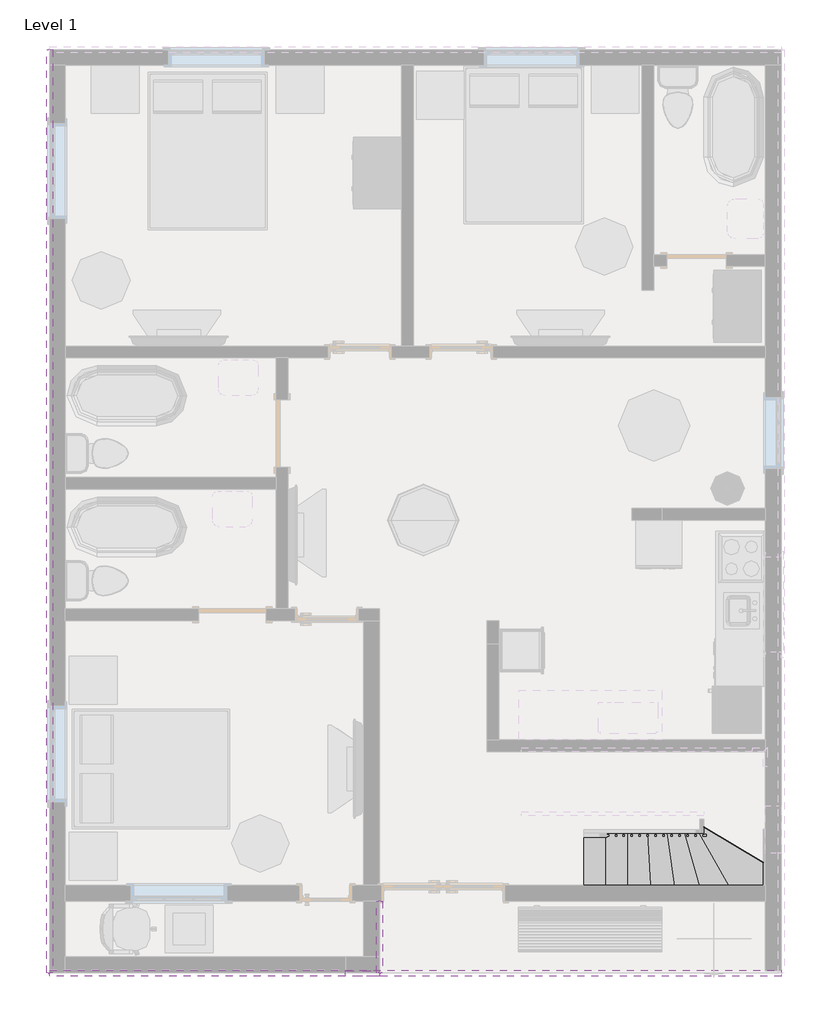
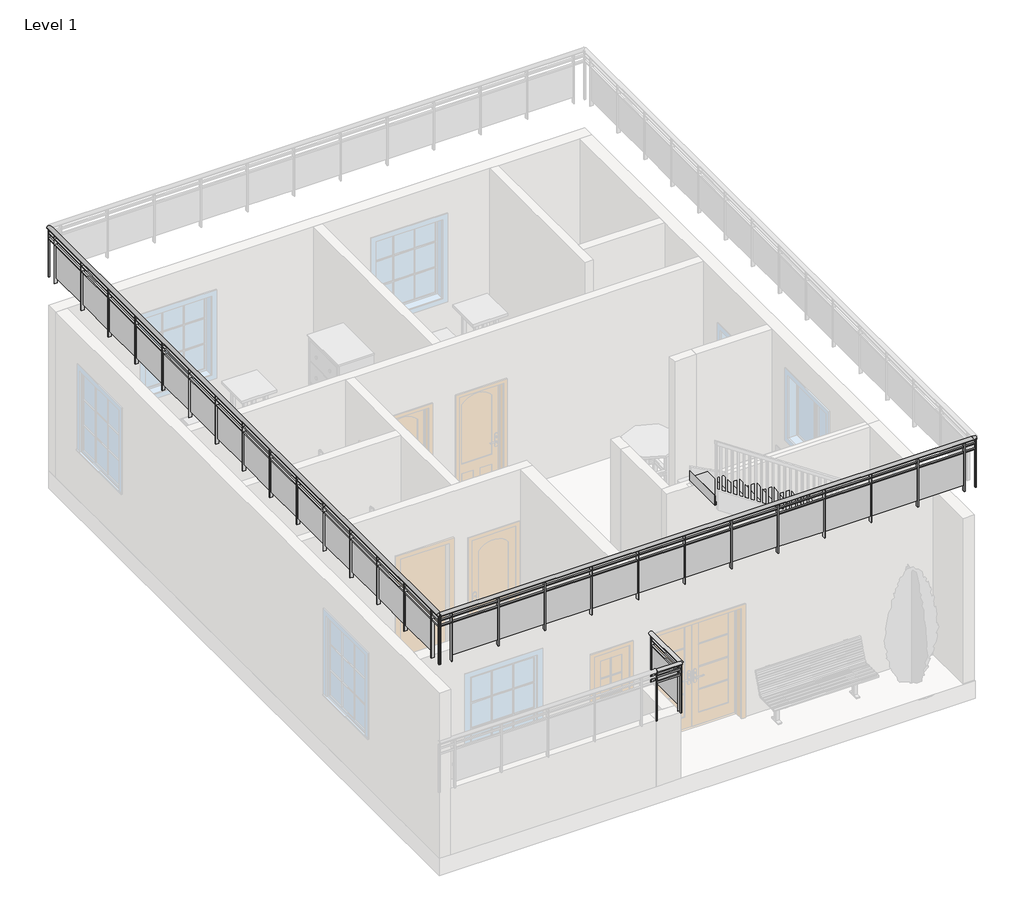
# One storey, part 2 of 4: 4 railings, 1 stair flight.
"""IFC4 building model written with IfcOpenShell, lengths in millimetres."""

from ifc_helpers import new_model, si_unit, point, frame, origin, place, context, project, spatial, polyline, ellipse_curve, trimmed, outline, extrude, transform, mapped, element, save
from ifc_brep_helpers import plane_surface, extruded_surface, advanced_brep
from components import stair_flight_7608b1ce

model = new_model("IFC4")

# Units and contexts
model_context = context("Model", 3, world=origin())
ifc_project = project(units=[si_unit("LENGTHUNIT", "METRE", prefix="MILLI")], contexts=[model_context])

# Site, building, storey
site = spatial("IfcSite", under=ifc_project)
building = spatial("IfcBuilding", under=site)
storey = spatial("IfcBuildingStorey", under=building, Name="Level 1", Elevation=0.0)

# Railings
placement = place(None, origin())
element("IfcRailing", 1, ObjectType="Glass Panel - Bottom Fill", at=placement, inside=storey, context=model_context, shape_type="SolidModel", body=[
    advanced_brep(
    [(-20.3394177, -1651.5409676, 2133.6), (-20.3394177, -1727.7409676, 2133.6), (411.4605823, -1651.5409676, 2133.6), (411.4605823, -1727.7409676, 2133.6)],
    [
        (0, 1, ellipse_curve(frame((-20.3394177, -1689.6409676, 2133.6), z_axis=(-1.0, 0.0, 0.0), x_axis=(0.0, -1.0, 0.0)), 38.1, 28.575)),
        (1, 0, ellipse_curve(frame((-20.3394177, -1689.6409676, 2133.6), z_axis=(-1.0, 0.0, 0.0), x_axis=(0.0, -1.0, 0.0)), 38.1, 28.575)),
        (2, 3, ellipse_curve(frame((411.4605823, -1689.6409676, 2133.6), z_axis=(1.0, 0.0, 0.0), x_axis=(0.0, -1.0, 0.0)), 38.1, 28.575)),
        (3, 2, ellipse_curve(frame((411.4605823, -1689.6409676, 2133.6), z_axis=(1.0, 0.0, 0.0), x_axis=(0.0, -1.0, 0.0)), 38.1, 28.575)),
        (0, 2),
        (3, 1),
    ],
    [
        plane_surface(frame((-20.3394177, -1689.6409676, 2133.6), z_axis=(-1.0, 0.0, 0.0), x_axis=(0.0, 1.0, 0.0))),
        plane_surface(frame((411.4605823, -1689.6409676, 2133.6), z_axis=(1.0, 0.0, 0.0), x_axis=(0.0, 1.0, 0.0))),
        extruded_surface(trimmed(ellipse_curve(frame((411.4605823, -1689.6409676, 2133.6), z_axis=(-1.0, 0.0, 0.0), x_axis=(0.0, -1.0, 0.0)), 38.1, 28.575), [point((411.4605823, -1651.5409676, 2133.6))], [point((411.4605823, -1727.7409676, 2133.6))], True, "CARTESIAN"), (-431.8, 0.0, 0.0), 431.8),
        extruded_surface(trimmed(ellipse_curve(frame((411.4605823, -1689.6409676, 2133.6), z_axis=(-1.0, 0.0, 0.0), x_axis=(0.0, -1.0, 0.0)), 38.1, 28.575), [point((411.4605823, -1727.7409676, 2133.6))], [point((411.4605823, -1651.5409676, 2133.6))], True, "CARTESIAN"), (-431.8, 0.0, 0.0), 431.8),
    ],
    [
        (0, [[1, 2]]),
        (1, [[3, 4]]),
        (2, [[-1, 5, -4, 6]]),
        (3, [[-2, -6, -3, -5]]),
    ],
),
    extrude(outline(polyline([(-20.3394177, -1702.3409676), (-20.3394177, -1676.9409676), (411.4605823, -1676.9409676), (411.4605823, -1702.3409676), (-20.3394177, -1702.3409676)])), frame((0.0, 0.0, 2019.3), z_axis=(0.0, 0.0, 1.0), x_axis=(1.0, 0.0, 0.0)), (0.0, 0.0, 1.0), 25.4),
    extrude(outline(polyline([(-20.3394177, -1702.3409676), (-20.3394177, -1676.9409676), (411.4605823, -1676.9409676), (411.4605823, -1702.3409676), (-20.3394177, -1702.3409676)])), frame((0.0, 0.0, 1917.7), z_axis=(0.0, 0.0, 1.0), x_axis=(1.0, 0.0, 0.0)), (0.0, 0.0, 1.0), 25.4),
    extrude(outline(polyline([(398.7605823, -1699.1659676), (398.7605823, -1680.1159676), (417.8105823, -1680.1159676), (417.8105823, -1699.1659676), (398.7605823, -1699.1659676)])), frame((0.0, 0.0, 1219.2), z_axis=(0.0, 0.0, 1.0), x_axis=(1.0, 0.0, 0.0)), (0.0, 0.0, 1.0), 885.6788223),
    extrude(outline(polyline([(-26.6894177, -1699.1659676), (-26.6894177, -1680.1159676), (-7.6394177, -1680.1159676), (-7.6394177, -1699.1659676), (-26.6894177, -1699.1659676)])), frame((0.0, 0.0, 1219.2), z_axis=(0.0, 0.0, 1.0), x_axis=(1.0, 0.0, 0.0)), (0.0, 0.0, 1.0), 885.6788223),
])
element("IfcRailing", 2, ObjectType="Glass Panel - Bottom Fill", at=placement, inside=storey, context=model_context, shape_type="SolidModel", body=[
    advanced_brep(
    [(376.5355823, -1680.1159676, 2133.6), (452.7355823, -1680.1159676, 2133.6), (376.5355823, -765.7159676, 2133.6), (452.7355823, -765.7159676, 2133.6)],
    [
        (0, 1, ellipse_curve(frame((414.6355823, -1680.1159676, 2133.6), z_axis=(0.0, -1.0, 0.0), x_axis=(1.0, 0.0, 0.0)), 38.1, 28.575)),
        (1, 0, ellipse_curve(frame((414.6355823, -1680.1159676, 2133.6), z_axis=(0.0, -1.0, 0.0), x_axis=(1.0, 0.0, 0.0)), 38.1, 28.575)),
        (2, 3, ellipse_curve(frame((414.6355823, -765.7159676, 2133.6), z_axis=(0.0, 1.0, 0.0), x_axis=(1.0, 0.0, 0.0)), 38.1, 28.575)),
        (3, 2, ellipse_curve(frame((414.6355823, -765.7159676, 2133.6), z_axis=(0.0, 1.0, 0.0), x_axis=(1.0, 0.0, 0.0)), 38.1, 28.575)),
        (0, 2),
        (3, 1),
    ],
    [
        plane_surface(frame((414.6355823, -1680.1159676, 2133.6), z_axis=(0.0, -1.0, 0.0), x_axis=(0.0, 0.0, 1.0))),
        plane_surface(frame((414.6355823, -765.7159676, 2133.6), z_axis=(0.0, 1.0, 0.0), x_axis=(0.0, 0.0, 1.0))),
        extruded_surface(trimmed(ellipse_curve(frame((414.6355823, -765.7159676, 2133.6), z_axis=(0.0, -1.0, 0.0), x_axis=(1.0, 0.0, 0.0)), 38.1, 28.575), [point((376.5355823, -765.7159676, 2133.6))], [point((452.7355823, -765.7159676, 2133.6))], True, "CARTESIAN"), (0.0, -914.4, 0.0), 914.4),
        extruded_surface(trimmed(ellipse_curve(frame((414.6355823, -765.7159676, 2133.6), z_axis=(0.0, -1.0, 0.0), x_axis=(1.0, 0.0, 0.0)), 38.1, 28.575), [point((452.7355823, -765.7159676, 2133.6))], [point((376.5355823, -765.7159676, 2133.6))], True, "CARTESIAN"), (0.0, -914.4, 0.0), 914.4),
    ],
    [
        (0, [[1, 2]]),
        (1, [[3, 4]]),
        (2, [[-1, 5, -4, 6]]),
        (3, [[-2, -6, -3, -5]]),
    ],
),
    extrude(outline(polyline([(427.3355823, -1680.1159676), (401.9355823, -1680.1159676), (401.9355823, -765.7159676), (427.3355823, -765.7159676), (427.3355823, -1680.1159676)])), frame((0.0, 0.0, 2019.3), z_axis=(0.0, 0.0, 1.0), x_axis=(1.0, 0.0, 0.0)), (0.0, 0.0, 1.0), 25.4),
    extrude(outline(polyline([(427.3355823, -1680.1159676), (401.9355823, -1680.1159676), (401.9355823, -765.7159676), (427.3355823, -765.7159676), (427.3355823, -1680.1159676)])), frame((0.0, 0.0, 1917.7), z_axis=(0.0, 0.0, 1.0), x_axis=(1.0, 0.0, 0.0)), (0.0, 0.0, 1.0), 25.4),
    extrude(outline(polyline([(440.0355823, -822.8659676), (389.2355823, -822.8659676), (389.2355823, -810.1659676), (440.0355823, -810.1659676), (440.0355823, -822.8659676)])), frame((0.0, 0.0, 1219.2), z_axis=(0.0, 0.0, 1.0), x_axis=(1.0, 0.0, 0.0)), (0.0, 0.0, 1.0), 885.6788223),
    extrude(outline(polyline([(408.1004253, -1629.3159676), (408.1004253, -816.5159676), (414.4504253, -816.5159676), (414.4504253, -1629.3159676), (408.1004253, -1629.3159676)])), frame((0.0, 0.0, 1320.8), z_axis=(0.0, 0.0, 1.0), x_axis=(1.0, 0.0, 0.0)), (0.0, 0.0, 1.0), 596.9),
    extrude(outline(polyline([(440.0355823, -1635.6659676), (389.2355823, -1635.6659676), (389.2355823, -1622.9659676), (440.0355823, -1622.9659676), (440.0355823, -1635.6659676)])), frame((0.0, 0.0, 1219.2), z_axis=(0.0, 0.0, 1.0), x_axis=(1.0, 0.0, 0.0)), (0.0, 0.0, 1.0), 885.6788223),
    extrude(outline(polyline([(424.1605823, -778.4159676), (405.1105823, -778.4159676), (405.1105823, -759.3659676), (424.1605823, -759.3659676), (424.1605823, -778.4159676)])), frame((0.0, 0.0, 1219.2), z_axis=(0.0, 0.0, 1.0), x_axis=(1.0, 0.0, 0.0)), (0.0, 0.0, 1.0), 885.6788223),
    extrude(outline(polyline([(424.1605823, -1686.4659676), (405.1105823, -1686.4659676), (405.1105823, -1667.4159676), (424.1605823, -1667.4159676), (424.1605823, -1686.4659676)])), frame((0.0, 0.0, 1219.2), z_axis=(0.0, 0.0, 1.0), x_axis=(1.0, 0.0, 0.0)), (0.0, 0.0, 1.0), 885.6788223),
])
element("IfcRailing", 3, ObjectType="Glass Panel - Bottom Fill", at=placement, inside=storey, context=model_context, shape_type="SolidModel", body=[
    advanced_brep(
    [(-3763.6644177, 10105.4840324, 4495.8), (-3839.8644177, 10105.4840324, 4495.8), (-3763.6644177, -1680.1159676, 4495.8), (-3839.8644177, -1680.1159676, 4495.8)],
    [
        (0, 1, ellipse_curve(frame((-3801.7644177, 10105.4840324, 4495.8), z_axis=(0.0, 1.0, 0.0), x_axis=(-1.0, 0.0, 0.0)), 38.1, 28.575)),
        (1, 0, ellipse_curve(frame((-3801.7644177, 10105.4840324, 4495.8), z_axis=(0.0, 1.0, 0.0), x_axis=(-1.0, 0.0, 0.0)), 38.1, 28.575)),
        (2, 3, ellipse_curve(frame((-3801.7644177, -1680.1159676, 4495.8), z_axis=(0.0, -1.0, 0.0), x_axis=(-1.0, 0.0, 0.0)), 38.1, 28.575)),
        (3, 2, ellipse_curve(frame((-3801.7644177, -1680.1159676, 4495.8), z_axis=(0.0, -1.0, 0.0), x_axis=(-1.0, 0.0, 0.0)), 38.1, 28.575)),
        (0, 2),
        (3, 1),
    ],
    [
        plane_surface(frame((-3801.7644177, 10105.4840324, 4495.8), z_axis=(0.0, 1.0, 0.0), x_axis=(0.0, 0.0, -1.0))),
        plane_surface(frame((-3801.7644177, -1680.1159676, 4495.8), z_axis=(0.0, -1.0, 0.0), x_axis=(0.0, 0.0, -1.0))),
        extruded_surface(trimmed(ellipse_curve(frame((-3801.7644177, -1680.1159676, 4495.8), z_axis=(0.0, 1.0, 0.0), x_axis=(-1.0, 0.0, 0.0)), 38.1, 28.575), [point((-3763.6644177, -1680.1159676, 4495.8))], [point((-3839.8644177, -1680.1159676, 4495.8))], True, "CARTESIAN"), (0.0, 11785.6, 0.0), 11785.6),
        extruded_surface(trimmed(ellipse_curve(frame((-3801.7644177, -1680.1159676, 4495.8), z_axis=(0.0, 1.0, 0.0), x_axis=(-1.0, 0.0, 0.0)), 38.1, 28.575), [point((-3839.8644177, -1680.1159676, 4495.8))], [point((-3763.6644177, -1680.1159676, 4495.8))], True, "CARTESIAN"), (0.0, 11785.6, 0.0), 11785.6),
    ],
    [
        (0, [[1, 2]]),
        (1, [[3, 4]]),
        (2, [[-1, 5, -4, 6]]),
        (3, [[-2, -6, -3, -5]]),
    ],
),
    extrude(outline(polyline([(-3814.4644177, 10105.4840324), (-3789.0644177, 10105.4840324), (-3789.0644177, -1680.1159676), (-3814.4644177, -1680.1159676), (-3814.4644177, 10105.4840324)])), frame((0.0, 0.0, 4381.5), z_axis=(0.0, 0.0, 1.0), x_axis=(1.0, 0.0, 0.0)), (0.0, 0.0, 1.0), 25.4),
    extrude(outline(polyline([(-3814.4644177, 10105.4840324), (-3789.0644177, 10105.4840324), (-3789.0644177, -1680.1159676), (-3814.4644177, -1680.1159676), (-3814.4644177, 10105.4840324)])), frame((0.0, 0.0, 4279.9), z_axis=(0.0, 0.0, 1.0), x_axis=(1.0, 0.0, 0.0)), (0.0, 0.0, 1.0), 25.4),
    extrude(outline(polyline([(-3827.1644177, -1470.5659676), (-3776.3644177, -1470.5659676), (-3776.3644177, -1483.2659676), (-3827.1644177, -1483.2659676), (-3827.1644177, -1470.5659676)])), frame((0.0, 0.0, 3581.4), z_axis=(0.0, 0.0, 1.0), x_axis=(1.0, 0.0, 0.0)), (0.0, 0.0, 1.0), 885.6788223),
    extrude(outline(polyline([(-3795.2292607, -664.1159676), (-3795.2292607, -1476.9159676), (-3801.5792607, -1476.9159676), (-3801.5792607, -664.1159676), (-3795.2292607, -664.1159676)])), frame((0.0, 0.0, 3683.0), z_axis=(0.0, 0.0, 1.0), x_axis=(1.0, 0.0, 0.0)), (0.0, 0.0, 1.0), 596.9),
    extrude(outline(polyline([(-3827.1644177, -657.7659676), (-3776.3644177, -657.7659676), (-3776.3644177, -670.4659676), (-3827.1644177, -670.4659676), (-3827.1644177, -657.7659676)])), frame((0.0, 0.0, 3581.4), z_axis=(0.0, 0.0, 1.0), x_axis=(1.0, 0.0, 0.0)), (0.0, 0.0, 1.0), 885.6788223),
    extrude(outline(polyline([(-3795.2292607, 148.6840324), (-3795.2292607, -664.1159676), (-3801.5792607, -664.1159676), (-3801.5792607, 148.6840324), (-3795.2292607, 148.6840324)])), frame((0.0, 0.0, 3683.0), z_axis=(0.0, 0.0, 1.0), x_axis=(1.0, 0.0, 0.0)), (0.0, 0.0, 1.0), 596.9),
    extrude(outline(polyline([(-3827.1644177, 155.0340324), (-3776.3644177, 155.0340324), (-3776.3644177, 142.3340324), (-3827.1644177, 142.3340324), (-3827.1644177, 155.0340324)])), frame((0.0, 0.0, 3581.4), z_axis=(0.0, 0.0, 1.0), x_axis=(1.0, 0.0, 0.0)), (0.0, 0.0, 1.0), 885.6788223),
    extrude(outline(polyline([(-3795.2292607, 961.4840324), (-3795.2292607, 148.6840324), (-3801.5792607, 148.6840324), (-3801.5792607, 961.4840324), (-3795.2292607, 961.4840324)])), frame((0.0, 0.0, 3683.0), z_axis=(0.0, 0.0, 1.0), x_axis=(1.0, 0.0, 0.0)), (0.0, 0.0, 1.0), 596.9),
    extrude(outline(polyline([(-3827.1644177, 967.8340324), (-3776.3644177, 967.8340324), (-3776.3644177, 955.1340324), (-3827.1644177, 955.1340324), (-3827.1644177, 967.8340324)])), frame((0.0, 0.0, 3581.4), z_axis=(0.0, 0.0, 1.0), x_axis=(1.0, 0.0, 0.0)), (0.0, 0.0, 1.0), 885.6788223),
    extrude(outline(polyline([(-3795.2292607, 1774.2840324), (-3795.2292607, 961.4840324), (-3801.5792607, 961.4840324), (-3801.5792607, 1774.2840324), (-3795.2292607, 1774.2840324)])), frame((0.0, 0.0, 3683.0), z_axis=(0.0, 0.0, 1.0), x_axis=(1.0, 0.0, 0.0)), (0.0, 0.0, 1.0), 596.9),
    extrude(outline(polyline([(-3827.1644177, 1780.6340324), (-3776.3644177, 1780.6340324), (-3776.3644177, 1767.9340324), (-3827.1644177, 1767.9340324), (-3827.1644177, 1780.6340324)])), frame((0.0, 0.0, 3581.4), z_axis=(0.0, 0.0, 1.0), x_axis=(1.0, 0.0, 0.0)), (0.0, 0.0, 1.0), 885.6788223),
    extrude(outline(polyline([(-3795.2292607, 2587.0840324), (-3795.2292607, 1774.2840324), (-3801.5792607, 1774.2840324), (-3801.5792607, 2587.0840324), (-3795.2292607, 2587.0840324)])), frame((0.0, 0.0, 3683.0), z_axis=(0.0, 0.0, 1.0), x_axis=(1.0, 0.0, 0.0)), (0.0, 0.0, 1.0), 596.9),
    extrude(outline(polyline([(-3827.1644177, 2593.4340324), (-3776.3644177, 2593.4340324), (-3776.3644177, 2580.7340324), (-3827.1644177, 2580.7340324), (-3827.1644177, 2593.4340324)])), frame((0.0, 0.0, 3581.4), z_axis=(0.0, 0.0, 1.0), x_axis=(1.0, 0.0, 0.0)), (0.0, 0.0, 1.0), 885.6788223),
    extrude(outline(polyline([(-3795.2292607, 3399.8840324), (-3795.2292607, 2587.0840324), (-3801.5792607, 2587.0840324), (-3801.5792607, 3399.8840324), (-3795.2292607, 3399.8840324)])), frame((0.0, 0.0, 3683.0), z_axis=(0.0, 0.0, 1.0), x_axis=(1.0, 0.0, 0.0)), (0.0, 0.0, 1.0), 596.9),
    extrude(outline(polyline([(-3827.1644177, 3406.2340324), (-3776.3644177, 3406.2340324), (-3776.3644177, 3393.5340324), (-3827.1644177, 3393.5340324), (-3827.1644177, 3406.2340324)])), frame((0.0, 0.0, 3581.4), z_axis=(0.0, 0.0, 1.0), x_axis=(1.0, 0.0, 0.0)), (0.0, 0.0, 1.0), 885.6788223),
    extrude(outline(polyline([(-3795.2292607, 4212.6840324), (-3795.2292607, 3399.8840324), (-3801.5792607, 3399.8840324), (-3801.5792607, 4212.6840324), (-3795.2292607, 4212.6840324)])), frame((0.0, 0.0, 3683.0), z_axis=(0.0, 0.0, 1.0), x_axis=(1.0, 0.0, 0.0)), (0.0, 0.0, 1.0), 596.9),
    extrude(outline(polyline([(-3827.1644177, 4219.0340324), (-3776.3644177, 4219.0340324), (-3776.3644177, 4206.3340324), (-3827.1644177, 4206.3340324), (-3827.1644177, 4219.0340324)])), frame((0.0, 0.0, 3581.4), z_axis=(0.0, 0.0, 1.0), x_axis=(1.0, 0.0, 0.0)), (0.0, 0.0, 1.0), 885.6788223),
    extrude(outline(polyline([(-3795.2292607, 5025.4840324), (-3795.2292607, 4212.6840324), (-3801.5792607, 4212.6840324), (-3801.5792607, 5025.4840324), (-3795.2292607, 5025.4840324)])), frame((0.0, 0.0, 3683.0), z_axis=(0.0, 0.0, 1.0), x_axis=(1.0, 0.0, 0.0)), (0.0, 0.0, 1.0), 596.9),
    extrude(outline(polyline([(-3827.1644177, 5031.8340324), (-3776.3644177, 5031.8340324), (-3776.3644177, 5019.1340324), (-3827.1644177, 5019.1340324), (-3827.1644177, 5031.8340324)])), frame((0.0, 0.0, 3581.4), z_axis=(0.0, 0.0, 1.0), x_axis=(1.0, 0.0, 0.0)), (0.0, 0.0, 1.0), 885.6788223),
    extrude(outline(polyline([(-3795.2292607, 5838.2840324), (-3795.2292607, 5025.4840324), (-3801.5792607, 5025.4840324), (-3801.5792607, 5838.2840324), (-3795.2292607, 5838.2840324)])), frame((0.0, 0.0, 3683.0), z_axis=(0.0, 0.0, 1.0), x_axis=(1.0, 0.0, 0.0)), (0.0, 0.0, 1.0), 596.9),
    extrude(outline(polyline([(-3827.1644177, 5844.6340324), (-3776.3644177, 5844.6340324), (-3776.3644177, 5831.9340324), (-3827.1644177, 5831.9340324), (-3827.1644177, 5844.6340324)])), frame((0.0, 0.0, 3581.4), z_axis=(0.0, 0.0, 1.0), x_axis=(1.0, 0.0, 0.0)), (0.0, 0.0, 1.0), 885.6788223),
    extrude(outline(polyline([(-3795.2292607, 6651.0840324), (-3795.2292607, 5838.2840324), (-3801.5792607, 5838.2840324), (-3801.5792607, 6651.0840324), (-3795.2292607, 6651.0840324)])), frame((0.0, 0.0, 3683.0), z_axis=(0.0, 0.0, 1.0), x_axis=(1.0, 0.0, 0.0)), (0.0, 0.0, 1.0), 596.9),
    extrude(outline(polyline([(-3827.1644177, 6657.4340324), (-3776.3644177, 6657.4340324), (-3776.3644177, 6644.7340324), (-3827.1644177, 6644.7340324), (-3827.1644177, 6657.4340324)])), frame((0.0, 0.0, 3581.4), z_axis=(0.0, 0.0, 1.0), x_axis=(1.0, 0.0, 0.0)), (0.0, 0.0, 1.0), 885.6788223),
    extrude(outline(polyline([(-3795.2292607, 7463.8840324), (-3795.2292607, 6651.0840324), (-3801.5792607, 6651.0840324), (-3801.5792607, 7463.8840324), (-3795.2292607, 7463.8840324)])), frame((0.0, 0.0, 3683.0), z_axis=(0.0, 0.0, 1.0), x_axis=(1.0, 0.0, 0.0)), (0.0, 0.0, 1.0), 596.9),
    extrude(outline(polyline([(-3827.1644177, 7470.2340324), (-3776.3644177, 7470.2340324), (-3776.3644177, 7457.5340324), (-3827.1644177, 7457.5340324), (-3827.1644177, 7470.2340324)])), frame((0.0, 0.0, 3581.4), z_axis=(0.0, 0.0, 1.0), x_axis=(1.0, 0.0, 0.0)), (0.0, 0.0, 1.0), 885.6788223),
    extrude(outline(polyline([(-3795.2292607, 8276.6840324), (-3795.2292607, 7463.8840324), (-3801.5792607, 7463.8840324), (-3801.5792607, 8276.6840324), (-3795.2292607, 8276.6840324)])), frame((0.0, 0.0, 3683.0), z_axis=(0.0, 0.0, 1.0), x_axis=(1.0, 0.0, 0.0)), (0.0, 0.0, 1.0), 596.9),
    extrude(outline(polyline([(-3827.1644177, 8283.0340324), (-3776.3644177, 8283.0340324), (-3776.3644177, 8270.3340324), (-3827.1644177, 8270.3340324), (-3827.1644177, 8283.0340324)])), frame((0.0, 0.0, 3581.4), z_axis=(0.0, 0.0, 1.0), x_axis=(1.0, 0.0, 0.0)), (0.0, 0.0, 1.0), 885.6788223),
    extrude(outline(polyline([(-3795.2292607, 9089.4840324), (-3795.2292607, 8276.6840324), (-3801.5792607, 8276.6840324), (-3801.5792607, 9089.4840324), (-3795.2292607, 9089.4840324)])), frame((0.0, 0.0, 3683.0), z_axis=(0.0, 0.0, 1.0), x_axis=(1.0, 0.0, 0.0)), (0.0, 0.0, 1.0), 596.9),
    extrude(outline(polyline([(-3827.1644177, 9095.8340324), (-3776.3644177, 9095.8340324), (-3776.3644177, 9083.1340324), (-3827.1644177, 9083.1340324), (-3827.1644177, 9095.8340324)])), frame((0.0, 0.0, 3581.4), z_axis=(0.0, 0.0, 1.0), x_axis=(1.0, 0.0, 0.0)), (0.0, 0.0, 1.0), 885.6788223),
    extrude(outline(polyline([(-3795.2292607, 9902.2840324), (-3795.2292607, 9089.4840324), (-3801.5792607, 9089.4840324), (-3801.5792607, 9902.2840324), (-3795.2292607, 9902.2840324)])), frame((0.0, 0.0, 3683.0), z_axis=(0.0, 0.0, 1.0), x_axis=(1.0, 0.0, 0.0)), (0.0, 0.0, 1.0), 596.9),
    extrude(outline(polyline([(-3827.1644177, 9908.6340324), (-3776.3644177, 9908.6340324), (-3776.3644177, 9895.9340324), (-3827.1644177, 9895.9340324), (-3827.1644177, 9908.6340324)])), frame((0.0, 0.0, 3581.4), z_axis=(0.0, 0.0, 1.0), x_axis=(1.0, 0.0, 0.0)), (0.0, 0.0, 1.0), 885.6788223),
    extrude(outline(polyline([(-3811.2894177, -1667.4159676), (-3792.2394177, -1667.4159676), (-3792.2394177, -1686.4659676), (-3811.2894177, -1686.4659676), (-3811.2894177, -1667.4159676)])), frame((0.0, 0.0, 3581.4), z_axis=(0.0, 0.0, 1.0), x_axis=(1.0, 0.0, 0.0)), (0.0, 0.0, 1.0), 885.6788223),
    extrude(outline(polyline([(-3811.2894177, 10111.8340324), (-3792.2394177, 10111.8340324), (-3792.2394177, 10092.7840324), (-3811.2894177, 10092.7840324), (-3811.2894177, 10111.8340324)])), frame((0.0, 0.0, 3581.4), z_axis=(0.0, 0.0, 1.0), x_axis=(1.0, 0.0, 0.0)), (0.0, 0.0, 1.0), 885.6788223),
])
element("IfcRailing", 4, ObjectType="Glass Panel - Bottom Fill", at=placement, inside=storey, context=model_context, shape_type="SolidModel", body=[
    advanced_brep(
    [(-3798.5894177, -1651.5409676, 4495.8), (-3798.5894177, -1727.7409676, 4495.8), (5548.6105823, -1651.5409676, 4495.8), (5548.6105823, -1727.7409676, 4495.8)],
    [
        (0, 1, ellipse_curve(frame((-3798.5894177, -1689.6409676, 4495.8), z_axis=(-1.0, 0.0, 0.0), x_axis=(0.0, -1.0, 0.0)), 38.1, 28.575)),
        (1, 0, ellipse_curve(frame((-3798.5894177, -1689.6409676, 4495.8), z_axis=(-1.0, 0.0, 0.0), x_axis=(0.0, -1.0, 0.0)), 38.1, 28.575)),
        (2, 3, ellipse_curve(frame((5548.6105823, -1689.6409676, 4495.8), z_axis=(1.0, 0.0, 0.0), x_axis=(0.0, -1.0, 0.0)), 38.1, 28.575)),
        (3, 2, ellipse_curve(frame((5548.6105823, -1689.6409676, 4495.8), z_axis=(1.0, 0.0, 0.0), x_axis=(0.0, -1.0, 0.0)), 38.1, 28.575)),
        (0, 2),
        (3, 1),
    ],
    [
        plane_surface(frame((-3798.5894177, -1689.6409676, 4495.8), z_axis=(-1.0, 0.0, 0.0), x_axis=(0.0, 1.0, 0.0))),
        plane_surface(frame((5548.6105823, -1689.6409676, 4495.8), z_axis=(1.0, 0.0, 0.0), x_axis=(0.0, 1.0, 0.0))),
        extruded_surface(trimmed(ellipse_curve(frame((5548.6105823, -1689.6409676, 4495.8), z_axis=(-1.0, 0.0, 0.0), x_axis=(0.0, -1.0, 0.0)), 38.1, 28.575), [point((5548.6105823, -1651.5409676, 4495.8))], [point((5548.6105823, -1727.7409676, 4495.8))], True, "CARTESIAN"), (-9347.2, 0.0, 0.0), 9347.2),
        extruded_surface(trimmed(ellipse_curve(frame((5548.6105823, -1689.6409676, 4495.8), z_axis=(-1.0, 0.0, 0.0), x_axis=(0.0, -1.0, 0.0)), 38.1, 28.575), [point((5548.6105823, -1727.7409676, 4495.8))], [point((5548.6105823, -1651.5409676, 4495.8))], True, "CARTESIAN"), (-9347.2, 0.0, 0.0), 9347.2),
    ],
    [
        (0, [[1, 2]]),
        (1, [[3, 4]]),
        (2, [[-1, 5, -4, 6]]),
        (3, [[-2, -6, -3, -5]]),
    ],
),
    extrude(outline(polyline([(-3798.5894177, -1702.3409676), (-3798.5894177, -1676.9409676), (5548.6105823, -1676.9409676), (5548.6105823, -1702.3409676), (-3798.5894177, -1702.3409676)])), frame((0.0, 0.0, 4381.5), z_axis=(0.0, 0.0, 1.0), x_axis=(1.0, 0.0, 0.0)), (0.0, 0.0, 1.0), 25.4),
    extrude(outline(polyline([(-3798.5894177, -1702.3409676), (-3798.5894177, -1676.9409676), (5548.6105823, -1676.9409676), (5548.6105823, -1702.3409676), (-3798.5894177, -1702.3409676)])), frame((0.0, 0.0, 4279.9), z_axis=(0.0, 0.0, 1.0), x_axis=(1.0, 0.0, 0.0)), (0.0, 0.0, 1.0), 25.4),
    extrude(outline(polyline([(5339.0605823, -1715.0409676), (5339.0605823, -1664.2409676), (5351.7605823, -1664.2409676), (5351.7605823, -1715.0409676), (5339.0605823, -1715.0409676)])), frame((0.0, 0.0, 3581.4), z_axis=(0.0, 0.0, 1.0), x_axis=(1.0, 0.0, 0.0)), (0.0, 0.0, 1.0), 885.6788223),
    extrude(outline(polyline([(4532.6105823, -1683.1058106), (5345.4105823, -1683.1058106), (5345.4105823, -1689.4558106), (4532.6105823, -1689.4558106), (4532.6105823, -1683.1058106)])), frame((0.0, 0.0, 3683.0), z_axis=(0.0, 0.0, 1.0), x_axis=(1.0, 0.0, 0.0)), (0.0, 0.0, 1.0), 596.9),
    extrude(outline(polyline([(4526.2605823, -1715.0409676), (4526.2605823, -1664.2409676), (4538.9605823, -1664.2409676), (4538.9605823, -1715.0409676), (4526.2605823, -1715.0409676)])), frame((0.0, 0.0, 3581.4), z_axis=(0.0, 0.0, 1.0), x_axis=(1.0, 0.0, 0.0)), (0.0, 0.0, 1.0), 885.6788223),
    extrude(outline(polyline([(3719.8105823, -1683.1058106), (4532.6105823, -1683.1058106), (4532.6105823, -1689.4558106), (3719.8105823, -1689.4558106), (3719.8105823, -1683.1058106)])), frame((0.0, 0.0, 3683.0), z_axis=(0.0, 0.0, 1.0), x_axis=(1.0, 0.0, 0.0)), (0.0, 0.0, 1.0), 596.9),
    extrude(outline(polyline([(3713.4605823, -1715.0409676), (3713.4605823, -1664.2409676), (3726.1605823, -1664.2409676), (3726.1605823, -1715.0409676), (3713.4605823, -1715.0409676)])), frame((0.0, 0.0, 3581.4), z_axis=(0.0, 0.0, 1.0), x_axis=(1.0, 0.0, 0.0)), (0.0, 0.0, 1.0), 885.6788223),
    extrude(outline(polyline([(2907.0105823, -1683.1058106), (3719.8105823, -1683.1058106), (3719.8105823, -1689.4558106), (2907.0105823, -1689.4558106), (2907.0105823, -1683.1058106)])), frame((0.0, 0.0, 3683.0), z_axis=(0.0, 0.0, 1.0), x_axis=(1.0, 0.0, 0.0)), (0.0, 0.0, 1.0), 596.9),
    extrude(outline(polyline([(2900.6605823, -1715.0409676), (2900.6605823, -1664.2409676), (2913.3605823, -1664.2409676), (2913.3605823, -1715.0409676), (2900.6605823, -1715.0409676)])), frame((0.0, 0.0, 3581.4), z_axis=(0.0, 0.0, 1.0), x_axis=(1.0, 0.0, 0.0)), (0.0, 0.0, 1.0), 885.6788223),
    extrude(outline(polyline([(2094.2105823, -1683.1058106), (2907.0105823, -1683.1058106), (2907.0105823, -1689.4558106), (2094.2105823, -1689.4558106), (2094.2105823, -1683.1058106)])), frame((0.0, 0.0, 3683.0), z_axis=(0.0, 0.0, 1.0), x_axis=(1.0, 0.0, 0.0)), (0.0, 0.0, 1.0), 596.9),
    extrude(outline(polyline([(2087.8605823, -1715.0409676), (2087.8605823, -1664.2409676), (2100.5605823, -1664.2409676), (2100.5605823, -1715.0409676), (2087.8605823, -1715.0409676)])), frame((0.0, 0.0, 3581.4), z_axis=(0.0, 0.0, 1.0), x_axis=(1.0, 0.0, 0.0)), (0.0, 0.0, 1.0), 885.6788223),
    extrude(outline(polyline([(1281.4105823, -1683.1058106), (2094.2105823, -1683.1058106), (2094.2105823, -1689.4558106), (1281.4105823, -1689.4558106), (1281.4105823, -1683.1058106)])), frame((0.0, 0.0, 3683.0), z_axis=(0.0, 0.0, 1.0), x_axis=(1.0, 0.0, 0.0)), (0.0, 0.0, 1.0), 596.9),
    extrude(outline(polyline([(1275.0605823, -1715.0409676), (1275.0605823, -1664.2409676), (1287.7605823, -1664.2409676), (1287.7605823, -1715.0409676), (1275.0605823, -1715.0409676)])), frame((0.0, 0.0, 3581.4), z_axis=(0.0, 0.0, 1.0), x_axis=(1.0, 0.0, 0.0)), (0.0, 0.0, 1.0), 885.6788223),
    extrude(outline(polyline([(468.6105823, -1683.1058106), (1281.4105823, -1683.1058106), (1281.4105823, -1689.4558106), (468.6105823, -1689.4558106), (468.6105823, -1683.1058106)])), frame((0.0, 0.0, 3683.0), z_axis=(0.0, 0.0, 1.0), x_axis=(1.0, 0.0, 0.0)), (0.0, 0.0, 1.0), 596.9),
    extrude(outline(polyline([(462.2605823, -1715.0409676), (462.2605823, -1664.2409676), (474.9605823, -1664.2409676), (474.9605823, -1715.0409676), (462.2605823, -1715.0409676)])), frame((0.0, 0.0, 3581.4), z_axis=(0.0, 0.0, 1.0), x_axis=(1.0, 0.0, 0.0)), (0.0, 0.0, 1.0), 885.6788223),
    extrude(outline(polyline([(-344.1894177, -1683.1058106), (468.6105823, -1683.1058106), (468.6105823, -1689.4558106), (-344.1894177, -1689.4558106), (-344.1894177, -1683.1058106)])), frame((0.0, 0.0, 3683.0), z_axis=(0.0, 0.0, 1.0), x_axis=(1.0, 0.0, 0.0)), (0.0, 0.0, 1.0), 596.9),
    extrude(outline(polyline([(-350.5394177, -1715.0409676), (-350.5394177, -1664.2409676), (-337.8394177, -1664.2409676), (-337.8394177, -1715.0409676), (-350.5394177, -1715.0409676)])), frame((0.0, 0.0, 3581.4), z_axis=(0.0, 0.0, 1.0), x_axis=(1.0, 0.0, 0.0)), (0.0, 0.0, 1.0), 885.6788223),
    extrude(outline(polyline([(-1156.9894177, -1683.1058106), (-344.1894177, -1683.1058106), (-344.1894177, -1689.4558106), (-1156.9894177, -1689.4558106), (-1156.9894177, -1683.1058106)])), frame((0.0, 0.0, 3683.0), z_axis=(0.0, 0.0, 1.0), x_axis=(1.0, 0.0, 0.0)), (0.0, 0.0, 1.0), 596.9),
    extrude(outline(polyline([(-1163.3394177, -1715.0409676), (-1163.3394177, -1664.2409676), (-1150.6394177, -1664.2409676), (-1150.6394177, -1715.0409676), (-1163.3394177, -1715.0409676)])), frame((0.0, 0.0, 3581.4), z_axis=(0.0, 0.0, 1.0), x_axis=(1.0, 0.0, 0.0)), (0.0, 0.0, 1.0), 885.6788223),
    extrude(outline(polyline([(-1969.7894177, -1683.1058106), (-1156.9894177, -1683.1058106), (-1156.9894177, -1689.4558106), (-1969.7894177, -1689.4558106), (-1969.7894177, -1683.1058106)])), frame((0.0, 0.0, 3683.0), z_axis=(0.0, 0.0, 1.0), x_axis=(1.0, 0.0, 0.0)), (0.0, 0.0, 1.0), 596.9),
    extrude(outline(polyline([(-1976.1394177, -1715.0409676), (-1976.1394177, -1664.2409676), (-1963.4394177, -1664.2409676), (-1963.4394177, -1715.0409676), (-1976.1394177, -1715.0409676)])), frame((0.0, 0.0, 3581.4), z_axis=(0.0, 0.0, 1.0), x_axis=(1.0, 0.0, 0.0)), (0.0, 0.0, 1.0), 885.6788223),
    extrude(outline(polyline([(-2782.5894177, -1683.1058106), (-1969.7894177, -1683.1058106), (-1969.7894177, -1689.4558106), (-2782.5894177, -1689.4558106), (-2782.5894177, -1683.1058106)])), frame((0.0, 0.0, 3683.0), z_axis=(0.0, 0.0, 1.0), x_axis=(1.0, 0.0, 0.0)), (0.0, 0.0, 1.0), 596.9),
    extrude(outline(polyline([(-2788.9394177, -1715.0409676), (-2788.9394177, -1664.2409676), (-2776.2394177, -1664.2409676), (-2776.2394177, -1715.0409676), (-2788.9394177, -1715.0409676)])), frame((0.0, 0.0, 3581.4), z_axis=(0.0, 0.0, 1.0), x_axis=(1.0, 0.0, 0.0)), (0.0, 0.0, 1.0), 885.6788223),
    extrude(outline(polyline([(-3595.3894177, -1683.1058106), (-2782.5894177, -1683.1058106), (-2782.5894177, -1689.4558106), (-3595.3894177, -1689.4558106), (-3595.3894177, -1683.1058106)])), frame((0.0, 0.0, 3683.0), z_axis=(0.0, 0.0, 1.0), x_axis=(1.0, 0.0, 0.0)), (0.0, 0.0, 1.0), 596.9),
    extrude(outline(polyline([(-3601.7394177, -1715.0409676), (-3601.7394177, -1664.2409676), (-3589.0394177, -1664.2409676), (-3589.0394177, -1715.0409676), (-3601.7394177, -1715.0409676)])), frame((0.0, 0.0, 3581.4), z_axis=(0.0, 0.0, 1.0), x_axis=(1.0, 0.0, 0.0)), (0.0, 0.0, 1.0), 885.6788223),
    extrude(outline(polyline([(5535.9105823, -1699.1659676), (5535.9105823, -1680.1159676), (5554.9605823, -1680.1159676), (5554.9605823, -1699.1659676), (5535.9105823, -1699.1659676)])), frame((0.0, 0.0, 3581.4), z_axis=(0.0, 0.0, 1.0), x_axis=(1.0, 0.0, 0.0)), (0.0, 0.0, 1.0), 885.6788223),
    extrude(outline(polyline([(-3804.9394177, -1699.1659676), (-3804.9394177, -1680.1159676), (-3785.8894177, -1680.1159676), (-3785.8894177, -1699.1659676), (-3804.9394177, -1699.1659676)])), frame((0.0, 0.0, 3581.4), z_axis=(0.0, 0.0, 1.0), x_axis=(1.0, 0.0, 0.0)), (0.0, 0.0, 1.0), 885.6788223),
])

# Stair flight
stair_flight_shape = stair_flight_7608b1ce(model_context)
element("IfcStairFlight", 5, ObjectType="2\" Tread 1\" Nosing 1/4\" Riser", at=placement, inside=storey, context=model_context, shape_type="MappedRepresentation", body=[
    mapped(stair_flight_shape, transform((0.0, 0.0, 0.0), x_axis=(1.0, 0.0, 0.0), y_axis=(0.0, 1.0, 0.0), z_axis=(0.0, 0.0, 1.0))),
])

save(model, "model.ifc")

# Revit data of these elements
# Type "Glass Panel - Bottom Fill"
#   Assembly Code = "C2010400"
#   built-in parameter 1008612 = 0.0416667 (stored number, unit not read)
#   built-in parameter 1008611 = 0.0416667 (stored number, unit not read)
#   built-in parameter 1008609 = 0.333333 (stored number, unit not read)
#   built-in parameter 1008604 = 0.166667 (stored number, unit not read)
#   built-in parameter 1008603 = 0.166667 (stored number, unit not read)
#   Railing Height = 3' - 0"
#   built-in parameter 1008630 = 2
#   built-in parameter 1008610 = 2
#   built-in parameter 1008618 = Baluster - Square : 3/4"
# Element 1 (IfcRailing, "Glass Panel - Bottom Fill")
#   built-in parameter 1008621 = 4 (stored number, unit not read)
#   Phase Created = New Construction
# Element 2 (IfcRailing, "Glass Panel - Bottom Fill")
#   built-in parameter 1008621 = 4 (stored number, unit not read)
#   Phase Created = New Construction
#   Materials on its faces: "Glass"
# Elements 3, 4 (IfcRailing, "Glass Panel - Bottom Fill")
#   built-in parameter 1008621 = 11.75 (stored number, unit not read)
#   Phase Created = New Construction
#   Materials on its faces: "Glass"
# Element 5 (IfcStairFlight, "2\" Tread 1\" Nosing 1/4\" Riser")
#   Phase Created = New Construction
# Materials
#   "Glass": class "Glass", colour RGB 0 128 192, transparency 0.75, Description = "Soda Lime Glass", Cost = 0
